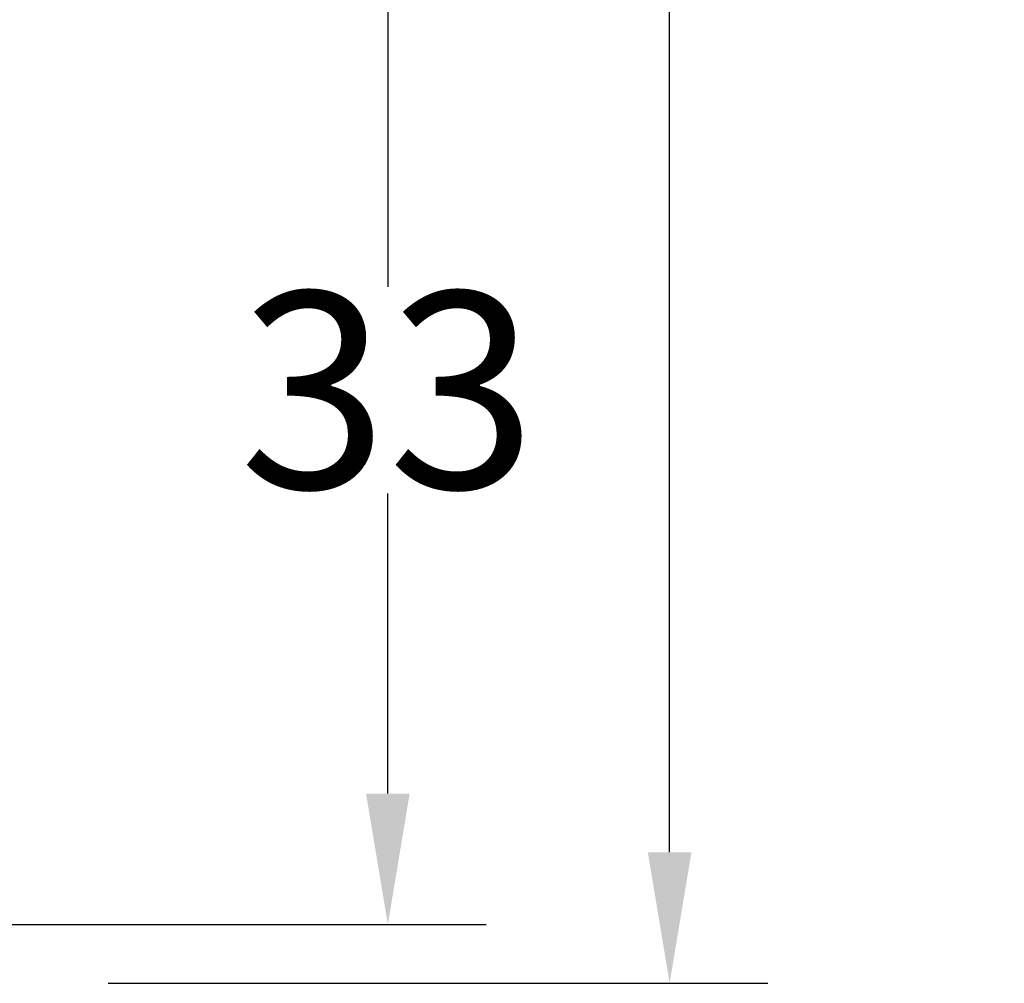
# Model space of a CAD drawing. Units: inches. Extents: x 89 to 490, y -59 to 378.
# Tile 16 of 20: x 460 to 490, y -27 to 3. Entities that reach past the tile are written whole.
import ezdxf

# ---------------------------------------------------------------- set-up
doc = ezdxf.new("R2010")
doc.units = ezdxf.units.IN
doc.header["$MEASUREMENT"] = 0
doc.layers.add('A-ANNO-DIMS', color=2, linetype='Continuous', lineweight=18)
doc.styles.get("Standard").update_dxf_attribs({"font": 'arial.ttf'})
doc.dimstyles.get("Standard").update_dxf_attribs({"dimtxt": 6, "dimasz": 4, "dimexe": 3, "dimexo": 3, "dimgap": 0.09, "dimtad": 0, "dimtih": 1, "dimtoh": 1, "dimdec": 1, "dimzin": 0, "dimdsep": 46, "dimlunit": 3, "dimtxsty": 'Standard', "dimcen": 0.09, "dimadec": 0, "dimazin": 0, "dimtfac": 1, "dimtdec": 1, "dimtofl": 0, "dimtmove": 0, "dimatfit": 3, "dimfxl": 1, "dimtolj": 1, "dimtzin": 0, "dimarcsym": 0})

# ---------------------------------------------------------------- blocks, each defined once
blk = doc.blocks.new('*D47')
at = {"layer": 'A-ANNO-DIMS', "color": 0, "lineweight": -2, "transparency": 16777216}
for p, q in [((448.739, 7.78), (473.983, 7.78)), ((470.983, 3.78), (470.983, -5.387)), ((470.983, -20.866), (470.983, -11.698)), ((448.739, -24.866), (473.983, -24.866))]:
    blk.add_line(p, q, dxfattribs=at)
at = {"layer": 'A-ANNO-DIMS', "color": 0, "transparency": 16777216}
for points in [[(470.316, 3.78), (471.65, 3.78), (470.983, 7.78)], [(470.316, -20.866), (471.65, -20.866), (470.983, -24.866)]]:
    blk.add_solid(points, dxfattribs=at)
at = {"layer": 'Defpoints', "color": 0, "transparency": 16777216}
for p in [(445.739, 7.78), (470.983, 7.78), (445.739, -24.866)]:
    blk.add_point(p, dxfattribs=at)
at = {"layer": 'A-ANNO-DIMS', "color": 0, "transparency": 16777216, "insert": (470.983, -8.543), "char_height": 6, "attachment_point": 5}
blk.add_mtext('\\A1;33', dxfattribs=at)
blk = doc.blocks.new('*D49')
at = {"layer": 'A-ANNO-DIMS', "color": 0, "lineweight": -2, "transparency": 16777216}
for p, q in [((462.441, 353.741), (482.591, 353.741)), ((479.591, 349.741), (479.591, 166.696)), ((479.591, -22.659), (479.591, 160.385)), ((462.441, -26.659), (482.591, -26.659))]:
    blk.add_line(p, q, dxfattribs=at)
at = {"layer": 'A-ANNO-DIMS', "color": 0, "transparency": 16777216}
for points in [[(478.925, 349.741), (480.258, 349.741), (479.591, 353.741)], [(478.925, -22.659), (480.258, -22.659), (479.591, -26.659)]]:
    blk.add_solid(points, dxfattribs=at)
at = {"layer": 'Defpoints', "color": 0, "transparency": 16777216}
for p in [(459.441, 353.741), (479.591, 353.741), (459.441, -26.659)]:
    blk.add_point(p, dxfattribs=at)
at = {"layer": 'A-ANNO-DIMS', "color": 0, "transparency": 16777216, "insert": (479.591, 163.541), "char_height": 6, "attachment_point": 5}
blk.add_mtext('\\A1;380.4', dxfattribs=at)

msp = doc.modelspace()

# ---------------------------------------------------------------- dimensions: what is measured, and where the dimension line sits
at = {"layer": 'A-ANNO-DIMS'}
for base, p1, p2, override, picture, middle in [((479.5914, 353.7413), (459.4414, -26.6594), (459.4414, 353.7413), {"dimdec": 1, "dimlfac": 1, "dimrnd": 0, "dimzin": 0, "dimdsep": 46, "dimlunit": 2}, '*D49', (479.5914, 163.5409)), ((470.9829, 7.78), (445.7386, -24.8656), (445.7386, 7.78), {"dimdec": 0, "dimlfac": 1, "dimrnd": 0, "dimzin": 0, "dimdsep": 46, "dimlunit": 2}, '*D47', (470.9829, -8.5428))]:
    dim = msp.add_linear_dim(base=base, p1=p1, p2=p2, angle=90, dimstyle='Standard', override=override, dxfattribs=at)
    dim.commit()
    dim.dimension.update_dxf_attribs({"geometry": picture, "text_midpoint": middle})

doc.saveas('drawing.dxf')
